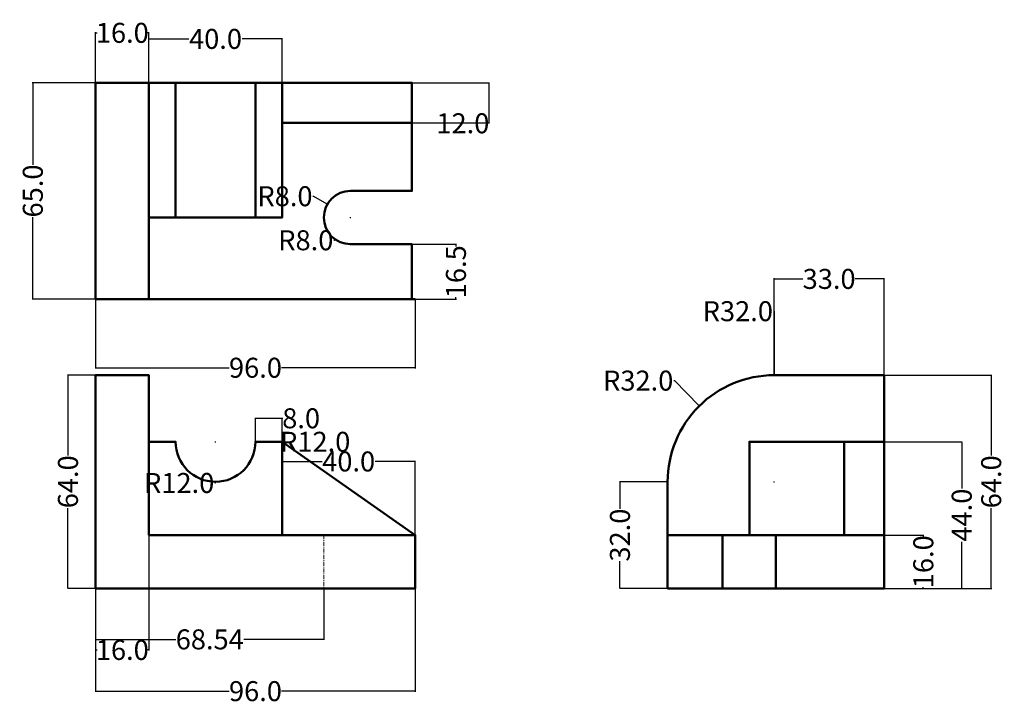
# Model space of a CAD drawing. Units: millimetres. Extents: x 2 to 298, y 17 to 222.
import ezdxf

# ---------------------------------------------------------------- set-up
doc = ezdxf.new("R2010")
doc.units = ezdxf.units.MM
doc.header["$MEASUREMENT"] = 0
doc.linetypes.add('CENTER', pattern=[2, 1.25, -0.25, 0.25, -0.25])
for name, color, linetype, lineweight in [('M-CNTR', 4, 'CENTER', 18), ('M-DIMS', 2, 'Continuous', 25), ('M-OUTL', 7, 'Continuous', 50)]:
    doc.layers.add(name, color=color, linetype=linetype, lineweight=lineweight)
doc.styles.get("Standard").update_dxf_attribs({"font": 'arial.ttf'})
doc.dimstyles.get("Standard").update_dxf_attribs({"dimtxt": 6, "dimasz": 0.18, "dimexe": 0.18, "dimexo": 0.0625, "dimgap": 0.09, "dimtad": 0, "dimtoh": 1, "dimdec": 1, "dimzin": 0, "dimdsep": 46, "dimtxsty": 'Standard', "dimcen": 0.09, "dimadec": 0, "dimazin": 0, "dimtfac": 1, "dimtdec": 1, "dimtofl": 0, "dimtmove": 0, "dimatfit": 3, "dimfxl": 1, "dimtolj": 1, "dimtzin": 0, "dimarcsym": 0})

# ---------------------------------------------------------------- blocks, each defined once
blk = doc.blocks.new('*D1')
at = {"layer": 'Defpoints', "color": 0, "transparency": 16777216}
for p in [(40.65, 218.17), (24.65, 203.2), (40.65, 203.2)]:
    blk.add_point(p, dxfattribs=at)
at = {"layer": 'M-DIMS', "color": 0, "lineweight": -2, "transparency": 16777216}
for p, q in [((24.65, 203.26), (24.65, 218.35)), ((24.83, 218.17), (25.06, 218.17)), ((40.47, 218.17), (40.24, 218.17)), ((40.65, 203.26), (40.65, 218.35))]:
    blk.add_line(p, q, dxfattribs=at)
at = {"layer": 'M-DIMS', "color": 0, "transparency": 16777216}
for points in [[(24.83, 218.2), (24.83, 218.14), (24.65, 218.17)], [(40.47, 218.2), (40.47, 218.14), (40.65, 218.17)]]:
    blk.add_solid(points, dxfattribs=at)
at = {"layer": 'M-DIMS', "color": 0, "transparency": 16777216, "insert": (32.65, 218.17), "char_height": 6, "attachment_point": 5}
blk.add_mtext('\\A1;16.0', dxfattribs=at)
blk = doc.blocks.new('*D2')
at = {"layer": 'Defpoints', "color": 0, "transparency": 16777216}
for p in [(80.65, 216.35), (40.65, 203.2), (80.65, 203.2)]:
    blk.add_point(p, dxfattribs=at)
at = {"layer": 'M-DIMS', "color": 0, "lineweight": -2, "transparency": 16777216}
for p, q in [((40.65, 203.26), (40.65, 216.53)), ((40.83, 216.35), (52.66, 216.35)), ((80.47, 216.35), (68.64, 216.35)), ((80.65, 203.26), (80.65, 216.53))]:
    blk.add_line(p, q, dxfattribs=at)
at = {"layer": 'M-DIMS', "color": 0, "transparency": 16777216}
for points in [[(40.83, 216.38), (40.83, 216.32), (40.65, 216.35)], [(80.47, 216.38), (80.47, 216.32), (80.65, 216.35)]]:
    blk.add_solid(points, dxfattribs=at)
at = {"layer": 'M-DIMS', "color": 0, "transparency": 16777216, "insert": (60.65, 216.35), "char_height": 6, "attachment_point": 5}
blk.add_mtext('\\A1;40.0', dxfattribs=at)
blk = doc.blocks.new('*D3')
at = {"layer": 'Defpoints', "color": 0, "transparency": 16777216}
for p in [(24.65, 203.2), (5.77, 138.2), (24.65, 138.2)]:
    blk.add_point(p, dxfattribs=at)
at = {"layer": 'M-DIMS', "color": 0, "lineweight": -2, "transparency": 16777216}
for p, q in [((24.59, 203.2), (5.59, 203.2)), ((5.77, 203.02), (5.77, 178.59)), ((5.77, 138.38), (5.77, 162.81)), ((24.59, 138.2), (5.59, 138.2))]:
    blk.add_line(p, q, dxfattribs=at)
at = {"layer": 'M-DIMS', "color": 0, "transparency": 16777216}
for points in [[(5.74, 203.02), (5.8, 203.02), (5.77, 203.2)], [(5.74, 138.38), (5.8, 138.38), (5.77, 138.2)]]:
    blk.add_solid(points, dxfattribs=at)
at = {"layer": 'M-DIMS', "color": 0, "transparency": 16777216, "insert": (5.77, 170.7), "char_height": 6, "attachment_point": 5, "rotation": 90}
blk.add_mtext('\\A1;65.0', dxfattribs=at)
blk = doc.blocks.new('*D4')
at = {"layer": 'Defpoints', "color": 0, "transparency": 16777216}
for p in [(24.65, 138.2), (120.65, 138.2), (120.65, 117.65)]:
    blk.add_point(p, dxfattribs=at)
at = {"layer": 'M-DIMS', "color": 0, "lineweight": -2, "transparency": 16777216}
for p, q in [((24.65, 138.14), (24.65, 117.47)), ((120.65, 138.14), (120.65, 117.47)), ((24.83, 117.65), (64.78, 117.65)), ((120.47, 117.65), (80.52, 117.65))]:
    blk.add_line(p, q, dxfattribs=at)
at = {"layer": 'M-DIMS', "color": 0, "transparency": 16777216}
for points in [[(24.83, 117.68), (24.83, 117.62), (24.65, 117.65)], [(120.47, 117.68), (120.47, 117.62), (120.65, 117.65)]]:
    blk.add_solid(points, dxfattribs=at)
at = {"layer": 'M-DIMS', "color": 0, "transparency": 16777216, "insert": (72.65, 117.65), "char_height": 6, "attachment_point": 5}
blk.add_mtext('\\A1;96.0', dxfattribs=at)
blk = doc.blocks.new('*D5')
at = {"layer": 'Defpoints', "color": 0, "transparency": 16777216}
for p in [(101.19, 162.73), (96.57, 156.2)]:
    blk.add_point(p, dxfattribs=at)
at = {"layer": 'M-DIMS', "color": 0, "lineweight": -2, "transparency": 16777216}
for p, q in [((101.1, 162.73), (101.28, 162.73)), ((101.19, 162.64), (101.19, 162.82)), ((96.18, 155.91), (96.36, 155.91)), ((96.36, 155.91), (96.47, 156.06))]:
    blk.add_line(p, q, dxfattribs=at)
at = {"layer": 'M-DIMS', "color": 0, "transparency": 16777216}
blk.add_solid([(96.44, 156.07), (96.49, 156.04), (96.57, 156.2)], dxfattribs=at)
at = {"layer": 'M-DIMS', "color": 0, "transparency": 16777216, "insert": (87.77, 155.91), "char_height": 6, "attachment_point": 5}
blk.add_mtext('\\A1;R8.0', dxfattribs=at)
blk = doc.blocks.new('*D6')
at = {"layer": 'Defpoints', "color": 0, "transparency": 16777216}
for p in [(119.65, 203.2), (119.65, 191.2), (142.72, 191.2)]:
    blk.add_point(p, dxfattribs=at)
at = {"layer": 'M-DIMS', "color": 0, "lineweight": -2, "transparency": 16777216}
for p, q in [((119.71, 203.2), (142.9, 203.2)), ((142.72, 203.02), (142.72, 191.38)), ((119.71, 191.2), (142.9, 191.2)), ((142.72, 191.02), (142.54, 191.02)), ((142.72, 191.2), (142.72, 191.02))]:
    blk.add_line(p, q, dxfattribs=at)
at = {"layer": 'M-DIMS', "color": 0, "transparency": 16777216}
for points in [[(142.69, 203.02), (142.75, 203.02), (142.72, 203.2)], [(142.69, 191.38), (142.75, 191.38), (142.72, 191.2)]]:
    blk.add_solid(points, dxfattribs=at)
at = {"layer": 'M-DIMS', "color": 0, "transparency": 16777216, "insert": (134.95, 191.02), "char_height": 6, "attachment_point": 5}
blk.add_mtext('\\A1;12.0', dxfattribs=at)
blk = doc.blocks.new('*D7')
at = {"layer": 'Defpoints', "color": 0, "transparency": 16777216}
for p in [(119.65, 154.73), (119.65, 138.2), (132.87, 138.2)]:
    blk.add_point(p, dxfattribs=at)
at = {"layer": 'M-DIMS', "color": 0, "lineweight": -2, "transparency": 16777216}
for p, q in [((119.71, 154.73), (133.05, 154.73)), ((132.87, 154.55), (132.87, 154.09)), ((119.71, 138.2), (133.05, 138.2)), ((132.87, 138.38), (132.87, 138.84))]:
    blk.add_line(p, q, dxfattribs=at)
at = {"layer": 'M-DIMS', "color": 0, "transparency": 16777216}
for points in [[(132.84, 154.55), (132.9, 154.55), (132.87, 154.73)], [(132.84, 138.38), (132.9, 138.38), (132.87, 138.2)]]:
    blk.add_solid(points, dxfattribs=at)
at = {"layer": 'M-DIMS', "color": 0, "transparency": 16777216, "insert": (132.87, 146.46), "char_height": 6, "attachment_point": 5, "rotation": 90}
blk.add_mtext('\\A1;16.5', dxfattribs=at)
blk = doc.blocks.new('*D8')
at = {"layer": 'Defpoints', "color": 0, "transparency": 16777216}
for p in [(24.65, 83.42), (40.65, 83.42), (40.65, 32.95)]:
    blk.add_point(p, dxfattribs=at)
at = {"layer": 'M-DIMS', "color": 0, "lineweight": -2, "transparency": 16777216}
for p, q in [((24.65, 83.35), (24.65, 32.77)), ((40.65, 83.35), (40.65, 32.77)), ((24.83, 32.95), (25.06, 32.95)), ((40.47, 32.95), (40.24, 32.95))]:
    blk.add_line(p, q, dxfattribs=at)
at = {"layer": 'M-DIMS', "color": 0, "transparency": 16777216}
for points in [[(24.83, 32.98), (24.83, 32.92), (24.65, 32.95)], [(40.47, 32.98), (40.47, 32.92), (40.65, 32.95)]]:
    blk.add_solid(points, dxfattribs=at)
at = {"layer": 'M-DIMS', "color": 0, "transparency": 16777216, "insert": (32.65, 32.95), "char_height": 6, "attachment_point": 5}
blk.add_mtext('\\A1;16.0', dxfattribs=at)
blk = doc.blocks.new('*D9')
at = {"layer": 'Defpoints', "color": 0, "transparency": 16777216}
for p in [(24.65, 115.42), (16.33, 51.42), (24.65, 51.42)]:
    blk.add_point(p, dxfattribs=at)
at = {"layer": 'M-DIMS', "color": 0, "lineweight": -2, "transparency": 16777216}
for p, q in [((24.59, 115.42), (16.15, 115.42)), ((16.33, 115.24), (16.33, 91.31)), ((16.33, 51.6), (16.33, 75.53)), ((24.59, 51.42), (16.15, 51.42))]:
    blk.add_line(p, q, dxfattribs=at)
at = {"layer": 'M-DIMS', "color": 0, "transparency": 16777216}
for points in [[(16.3, 115.24), (16.36, 115.24), (16.33, 115.42)], [(16.3, 51.6), (16.36, 51.6), (16.33, 51.42)]]:
    blk.add_solid(points, dxfattribs=at)
at = {"layer": 'M-DIMS', "color": 0, "transparency": 16777216, "insert": (16.33, 83.42), "char_height": 6, "attachment_point": 5, "rotation": 90}
blk.add_mtext('\\A1;64.0', dxfattribs=at)
blk = doc.blocks.new('*D10')
at = {"layer": 'Defpoints', "color": 0, "transparency": 16777216}
for p in [(60.65, 95.42), (60.65, 83.42)]:
    blk.add_point(p, dxfattribs=at)
at = {"layer": 'M-DIMS', "color": 0, "lineweight": -2, "transparency": 16777216}
for p, q in [((60.56, 95.42), (60.74, 95.42)), ((60.65, 95.33), (60.65, 95.51)), ((60.47, 83.06), (60.65, 83.06)), ((60.65, 83.06), (60.65, 83.24))]:
    blk.add_line(p, q, dxfattribs=at)
at = {"layer": 'M-DIMS', "color": 0, "transparency": 16777216}
blk.add_solid([(60.62, 83.24), (60.68, 83.24), (60.65, 83.42)], dxfattribs=at)
at = {"layer": 'M-DIMS', "color": 0, "transparency": 16777216, "insert": (49.73, 83.06), "char_height": 6, "attachment_point": 5}
blk.add_mtext('\\A1;R12.0', dxfattribs=at)
blk = doc.blocks.new('*D11')
at = {"layer": 'Defpoints', "color": 0, "transparency": 16777216}
for p in [(80.65, 102.48), (72.65, 95.42), (80.65, 95.42)]:
    blk.add_point(p, dxfattribs=at)
at = {"layer": 'M-DIMS', "color": 0, "lineweight": -2, "transparency": 16777216}
for p, q in [((72.65, 95.48), (72.65, 102.66)), ((72.83, 102.48), (80.47, 102.48)), ((80.65, 95.48), (80.65, 102.66)), ((80.65, 102.48), (80.83, 102.48))]:
    blk.add_line(p, q, dxfattribs=at)
at = {"layer": 'M-DIMS', "color": 0, "transparency": 16777216}
for points in [[(72.83, 102.51), (72.83, 102.45), (72.65, 102.48)], [(80.47, 102.51), (80.47, 102.45), (80.65, 102.48)]]:
    blk.add_solid(points, dxfattribs=at)
at = {"layer": 'M-DIMS', "color": 0, "transparency": 16777216, "insert": (86.37, 102.48), "char_height": 6, "attachment_point": 5}
blk.add_mtext('\\A1;8.0', dxfattribs=at)
blk = doc.blocks.new('*D12')
at = {"layer": 'Defpoints', "color": 0, "transparency": 16777216}
for p in [(120.65, 89.52), (80.65, 67.42), (120.65, 67.42)]:
    blk.add_point(p, dxfattribs=at)
at = {"layer": 'M-DIMS', "color": 0, "lineweight": -2, "transparency": 16777216}
for p, q in [((80.65, 67.48), (80.65, 89.7)), ((80.83, 89.52), (92.66, 89.52)), ((120.47, 89.52), (108.64, 89.52)), ((120.65, 67.48), (120.65, 89.7))]:
    blk.add_line(p, q, dxfattribs=at)
at = {"layer": 'M-DIMS', "color": 0, "transparency": 16777216}
for points in [[(80.83, 89.55), (80.83, 89.49), (80.65, 89.52)], [(120.47, 89.55), (120.47, 89.49), (120.65, 89.52)]]:
    blk.add_solid(points, dxfattribs=at)
at = {"layer": 'M-DIMS', "color": 0, "transparency": 16777216, "insert": (100.65, 89.52), "char_height": 6, "attachment_point": 5}
blk.add_mtext('\\A1;40.0', dxfattribs=at)
blk = doc.blocks.new('*D13')
at = {"layer": 'Defpoints', "color": 0, "transparency": 16777216}
for p in [(24.65, 51.42), (120.65, 51.42), (120.65, 20.58)]:
    blk.add_point(p, dxfattribs=at)
at = {"layer": 'M-DIMS', "color": 0, "lineweight": -2, "transparency": 16777216}
for p, q in [((24.65, 51.35), (24.65, 20.4)), ((120.65, 51.35), (120.65, 20.4)), ((24.83, 20.58), (64.78, 20.58)), ((120.47, 20.58), (80.52, 20.58))]:
    blk.add_line(p, q, dxfattribs=at)
at = {"layer": 'M-DIMS', "color": 0, "transparency": 16777216}
for points in [[(24.83, 20.61), (24.83, 20.55), (24.65, 20.58)], [(120.47, 20.61), (120.47, 20.55), (120.65, 20.58)]]:
    blk.add_solid(points, dxfattribs=at)
at = {"layer": 'M-DIMS', "color": 0, "transparency": 16777216, "insert": (72.65, 20.58), "char_height": 6, "attachment_point": 5}
blk.add_mtext('\\A1;96.0', dxfattribs=at)
blk = doc.blocks.new('*D14')
at = {"layer": 'Defpoints', "color": 0, "transparency": 16777216}
for p in [(261.46, 144.31), (228.46, 115.42), (261.46, 115.42)]:
    blk.add_point(p, dxfattribs=at)
at = {"layer": 'M-DIMS', "color": 0, "lineweight": -2, "transparency": 16777216}
for p, q in [((228.46, 115.48), (228.46, 144.49)), ((228.64, 144.31), (237.09, 144.31)), ((261.28, 144.31), (252.83, 144.31)), ((261.46, 115.48), (261.46, 144.49))]:
    blk.add_line(p, q, dxfattribs=at)
at = {"layer": 'M-DIMS', "color": 0, "transparency": 16777216}
for points in [[(228.64, 144.34), (228.64, 144.28), (228.46, 144.31)], [(261.28, 144.34), (261.28, 144.28), (261.46, 144.31)]]:
    blk.add_solid(points, dxfattribs=at)
at = {"layer": 'M-DIMS', "color": 0, "transparency": 16777216, "insert": (244.96, 144.31), "char_height": 6, "attachment_point": 5}
blk.add_mtext('\\A1;33.0', dxfattribs=at)
blk = doc.blocks.new('*D15')
at = {"layer": 'Defpoints', "color": 0, "transparency": 16777216}
for p in [(196.46, 83.42), (182.13, 51.42), (196.46, 51.42)]:
    blk.add_point(p, dxfattribs=at)
at = {"layer": 'M-DIMS', "color": 0, "lineweight": -2, "transparency": 16777216}
for p, q in [((196.39, 83.42), (181.95, 83.42)), ((182.13, 83.24), (182.13, 75.29)), ((182.13, 51.6), (182.13, 59.55)), ((196.39, 51.42), (181.95, 51.42))]:
    blk.add_line(p, q, dxfattribs=at)
at = {"layer": 'M-DIMS', "color": 0, "transparency": 16777216}
for points in [[(182.1, 83.24), (182.16, 83.24), (182.13, 83.42)], [(182.1, 51.6), (182.16, 51.6), (182.13, 51.42)]]:
    blk.add_solid(points, dxfattribs=at)
at = {"layer": 'M-DIMS', "color": 0, "transparency": 16777216, "insert": (182.13, 67.42), "char_height": 6, "attachment_point": 5, "rotation": 90}
blk.add_mtext('\\A1;32.0', dxfattribs=at)
blk = doc.blocks.new('*D16')
at = {"layer": 'Defpoints', "color": 0, "transparency": 16777216}
for p in [(261.46, 115.42), (261.46, 51.42), (293.64, 51.42)]:
    blk.add_point(p, dxfattribs=at)
at = {"layer": 'M-DIMS', "color": 0, "lineweight": -2, "transparency": 16777216}
for p, q in [((261.52, 115.42), (293.82, 115.42)), ((293.64, 115.24), (293.64, 91.31)), ((293.64, 51.6), (293.64, 75.53)), ((261.52, 51.42), (293.82, 51.42))]:
    blk.add_line(p, q, dxfattribs=at)
at = {"layer": 'M-DIMS', "color": 0, "transparency": 16777216}
for points in [[(293.61, 115.24), (293.67, 115.24), (293.64, 115.42)], [(293.61, 51.6), (293.67, 51.6), (293.64, 51.42)]]:
    blk.add_solid(points, dxfattribs=at)
at = {"layer": 'M-DIMS', "color": 0, "transparency": 16777216, "insert": (293.64, 83.42), "char_height": 6, "attachment_point": 5, "rotation": 90}
blk.add_mtext('\\A1;64.0', dxfattribs=at)
blk = doc.blocks.new('*D17')
at = {"layer": 'Defpoints', "color": 0, "transparency": 16777216}
for p in [(261.46, 95.42), (261.46, 51.42), (284.79, 51.42)]:
    blk.add_point(p, dxfattribs=at)
at = {"layer": 'M-DIMS', "color": 0, "lineweight": -2, "transparency": 16777216}
for p, q in [((261.52, 95.42), (284.97, 95.42)), ((284.79, 95.24), (284.79, 81.41)), ((284.79, 51.6), (284.79, 65.42)), ((261.52, 51.42), (284.97, 51.42))]:
    blk.add_line(p, q, dxfattribs=at)
at = {"layer": 'M-DIMS', "color": 0, "transparency": 16777216}
for points in [[(284.76, 95.24), (284.82, 95.24), (284.79, 95.42)], [(284.76, 51.6), (284.82, 51.6), (284.79, 51.42)]]:
    blk.add_solid(points, dxfattribs=at)
at = {"layer": 'M-DIMS', "color": 0, "transparency": 16777216, "insert": (284.79, 73.42), "char_height": 6, "attachment_point": 5, "rotation": 90}
blk.add_mtext('\\A1;44.0', dxfattribs=at)
blk = doc.blocks.new('*D18')
at = {"layer": 'Defpoints', "color": 0, "transparency": 16777216}
for p in [(261.46, 67.42), (261.46, 51.42), (273.25, 51.42)]:
    blk.add_point(p, dxfattribs=at)
at = {"layer": 'M-DIMS', "color": 0, "lineweight": -2, "transparency": 16777216}
for p, q in [((261.52, 67.42), (273.43, 67.42)), ((273.25, 67.24), (273.25, 67.01)), ((261.52, 51.42), (273.43, 51.42)), ((273.25, 51.6), (273.25, 51.83))]:
    blk.add_line(p, q, dxfattribs=at)
at = {"layer": 'M-DIMS', "color": 0, "transparency": 16777216}
for points in [[(273.22, 67.24), (273.28, 67.24), (273.25, 67.42)], [(273.22, 51.6), (273.28, 51.6), (273.25, 51.42)]]:
    blk.add_solid(points, dxfattribs=at)
at = {"layer": 'M-DIMS', "color": 0, "transparency": 16777216, "insert": (273.25, 59.42), "char_height": 6, "attachment_point": 5, "rotation": 90}
blk.add_mtext('\\A1;16.0', dxfattribs=at)
blk = doc.blocks.new('*D19')
at = {"layer": 'Defpoints', "color": 0, "transparency": 16777216}
for p in [(206, 106.21), (228.46, 83.42)]:
    blk.add_point(p, dxfattribs=at)
at = {"layer": 'M-DIMS', "color": 0, "lineweight": -2, "transparency": 16777216}
for p, q in [((198.36, 113.79), (198.54, 113.79)), ((198.54, 113.79), (205.87, 106.34)), ((228.37, 83.42), (228.55, 83.42)), ((228.46, 83.33), (228.46, 83.51))]:
    blk.add_line(p, q, dxfattribs=at)
at = {"layer": 'M-DIMS', "color": 0, "transparency": 16777216}
blk.add_solid([(205.89, 106.36), (205.85, 106.32), (206, 106.21)], dxfattribs=at)
at = {"layer": 'M-DIMS', "color": 0, "transparency": 16777216, "insert": (187.61, 113.79), "char_height": 6, "attachment_point": 5}
blk.add_mtext('\\A1;R32.0', dxfattribs=at)
blk = doc.blocks.new('*D20')
at = {"layer": 'Defpoints', "color": 0, "transparency": 16777216}
for p in [(24.65, 51.42), (93.19, 51.42), (93.19, 36.12)]:
    blk.add_point(p, dxfattribs=at)
at = {"layer": 'M-DIMS', "color": 0, "lineweight": -2, "transparency": 16777216}
for p, q in [((24.65, 51.35), (24.65, 35.94)), ((93.19, 51.35), (93.19, 35.94)), ((24.83, 36.12), (48.7, 36.12)), ((93.01, 36.12), (69.14, 36.12))]:
    blk.add_line(p, q, dxfattribs=at)
at = {"layer": 'M-DIMS', "color": 0, "transparency": 16777216}
for points in [[(24.83, 36.15), (24.83, 36.09), (24.65, 36.12)], [(93.01, 36.15), (93.01, 36.09), (93.19, 36.12)]]:
    blk.add_solid(points, dxfattribs=at)
at = {"layer": 'M-DIMS', "color": 0, "transparency": 16777216, "insert": (58.92, 36.12), "char_height": 6, "attachment_point": 5}
blk.add_mtext('\\A1;68.54', dxfattribs=at)
blk = doc.blocks.new('*D21')
at = {"layer": 'Defpoints', "color": 0, "transparency": 16777216}
for p in [(228.46, 115.42), (228.46, 83.42)]:
    blk.add_point(p, dxfattribs=at)
at = {"layer": 'M-DIMS', "color": 0, "lineweight": -2, "transparency": 16777216}
for p, q in [((228.28, 134.62), (228.46, 134.62)), ((228.46, 134.62), (228.46, 115.6)), ((228.37, 83.42), (228.55, 83.42)), ((228.46, 83.33), (228.46, 83.51))]:
    blk.add_line(p, q, dxfattribs=at)
at = {"layer": 'M-DIMS', "color": 0, "transparency": 16777216}
blk.add_solid([(228.49, 115.6), (228.43, 115.6), (228.46, 115.42)], dxfattribs=at)
at = {"layer": 'M-DIMS', "color": 0, "transparency": 16777216, "insert": (217.53, 134.62), "char_height": 6, "attachment_point": 5}
blk.add_mtext('\\A1;R32.0', dxfattribs=at)
blk = doc.blocks.new('*D22')
at = {"layer": 'Defpoints', "color": 0, "transparency": 16777216}
for p in [(60.65, 95.42), (72.65, 95.42)]:
    blk.add_point(p, dxfattribs=at)
at = {"layer": 'M-DIMS', "color": 0, "lineweight": -2, "transparency": 16777216}
for p, q in [((60.56, 95.42), (60.74, 95.42)), ((60.65, 95.33), (60.65, 95.51)), ((79.85, 95.42), (72.83, 95.42))]:
    blk.add_line(p, q, dxfattribs=at)
at = {"layer": 'M-DIMS', "color": 0, "transparency": 16777216}
blk.add_solid([(72.83, 95.45), (72.83, 95.39), (72.65, 95.42)], dxfattribs=at)
at = {"layer": 'M-DIMS', "color": 0, "transparency": 16777216, "insert": (90.59, 95.42), "char_height": 6, "attachment_point": 5}
blk.add_mtext('\\A1;R12.0', dxfattribs=at)
blk = doc.blocks.new('*D23')
at = {"layer": 'Defpoints', "color": 0, "transparency": 16777216}
for p in [(94.26, 166.73), (101.19, 162.73)]:
    blk.add_point(p, dxfattribs=at)
at = {"layer": 'M-DIMS', "color": 0, "lineweight": -2, "transparency": 16777216}
for p, q in [((89.92, 169.13), (90.1, 169.13)), ((90.1, 169.13), (94.11, 166.82)), ((101.1, 162.73), (101.28, 162.73)), ((101.19, 162.64), (101.19, 162.82))]:
    blk.add_line(p, q, dxfattribs=at)
at = {"layer": 'M-DIMS', "color": 0, "transparency": 16777216}
blk.add_solid([(94.12, 166.84), (94.09, 166.79), (94.26, 166.73)], dxfattribs=at)
at = {"layer": 'M-DIMS', "color": 0, "transparency": 16777216, "insert": (81.51, 169.13), "char_height": 6, "attachment_point": 5}
blk.add_mtext('\\A1;R8.0', dxfattribs=at)

msp = doc.modelspace()

# ---------------------------------------------------------------- linework, layer by layer
at = {"layer": 'M-CNTR'}
msp.add_line((93.192, 67.417), (93.192, 51.417), dxfattribs=at)
at = {"layer": 'M-OUTL'}
for p, q in [((40.649, 203.198), (40.649, 138.198)), ((72.649, 203.198), (72.649, 162.732)), ((119.649, 191.198), (80.649, 191.198)), ((249.456, 95.417), (249.456, 67.417)), ((196.456, 67.417), (261.456, 67.417)), ((212.956, 51.417), (212.956, 67.417)), ((228.956, 51.417), (228.956, 67.417))]:
    msp.add_line(p, q, dxfattribs=at)
for points in [[(120.649, 138.198), (24.649, 138.198), (24.649, 203.198), (119.649, 203.198), (119.649, 170.732), (101.192, 170.732, 1), (101.192, 154.732), (119.649, 154.732), (119.649, 138.198)], [(40.649, 95.417), (48.649, 95.417, 1), (72.649, 95.417), (80.649, 95.417)]]:
    msp.add_lwpolyline(points, format="xyb", dxfattribs=at)
for points in [[(40.649, 162.732), (48.649, 162.732), (80.649, 162.732), (80.649, 203.198)], [(48.649, 203.198), (48.649, 185.432), (48.649, 170.732), (48.649, 162.732)], [(80.649, 67.417), (80.649, 95.417), (120.649, 67.417), (120.649, 51.417), (24.649, 51.417), (24.649, 115.417), (40.649, 115.417), (40.649, 67.417), (120.649, 67.417)], [(261.456, 95.417), (236.497, 95.417), (220.997, 95.417), (220.997, 67.417)]]:
    msp.add_lwpolyline(points, dxfattribs=at)
msp.add_lwpolyline([(196.456, 51.417), (196.456, 83.417, -0.4142136), (228.456, 115.417), (261.456, 115.417), (261.456, 51.417)], format="xyb", close=True, dxfattribs=at)

# ---------------------------------------------------------------- dimensions: what is measured, and where the dimension line sits
at = {"layer": 'M-DIMS'}
for base, p1, p2, override, picture, middle in [((40.649, 218.173), (24.649, 203.198), (40.649, 203.198), {"dimclrd": 0, "dimclre": 0, "dimclrt": 0}, '*D1', (32.649, 218.173)), ((80.649, 216.351), (40.649, 203.198), (80.649, 203.198), {"dimclrd": 0, "dimclre": 0, "dimclrt": 0}, '*D2', (60.649, 216.351)), ((261.456, 144.313), (228.456, 115.417), (261.456, 115.417), {"dimclrd": 0, "dimclre": 0, "dimclrt": 0}, '*D14', (244.956, 144.313)), ((120.649, 117.651), (24.649, 138.198), (120.649, 138.198), {"dimclrd": 0, "dimclre": 0, "dimclrt": 0}, '*D4', (72.649, 117.651)), ((80.649, 102.478), (72.649, 95.417), (80.649, 95.417), {"dimclrd": 0, "dimclre": 0, "dimclrt": 0}, '*D11', (86.374, 102.478)), ((120.649, 89.515), (80.649, 67.417), (120.649, 67.417), {"dimclrd": 0, "dimclre": 0, "dimclrt": 0}, '*D12', (100.649, 89.515)), ((40.649, 32.95), (24.649, 83.417), (40.649, 83.417), {"dimclrd": 0, "dimclre": 0, "dimclrt": 0}, '*D8', (32.649, 32.95)), ((120.649, 20.576), (24.649, 51.417), (120.649, 51.417), {"dimclrd": 0, "dimclre": 0, "dimclrt": 0}, '*D13', (72.649, 20.576)), ((93.192, 36.117), (24.649, 51.417), (93.192, 51.417), {"dimdec": 2, "dimlfac": 1, "dimrnd": 0, "dimzin": 0, "dimdsep": 46, "dimlunit": 2}, '*D20', (58.921, 36.117))]:
    dim = msp.add_linear_dim(base=base, p1=p1, p2=p2, dimstyle='Standard', override=override, dxfattribs=at)
    dim.commit()
    dim.dimension.update_dxf_attribs({"geometry": picture, "text_midpoint": middle})
for base, p1, p2, picture, middle in [((5.768, 138.198), (24.649, 203.198), (24.649, 138.198), '*D3', (5.768, 170.698)), ((142.724, 191.198), (119.649, 203.198), (119.649, 191.198), '*D6', (134.954, 191.018)), ((132.869, 138.198), (119.649, 154.732), (119.649, 138.198), '*D7', (132.869, 146.465)), ((16.327, 51.417), (24.649, 115.417), (24.649, 51.417), '*D9', (16.327, 83.417)), ((293.644, 51.417), (261.456, 115.417), (261.456, 51.417), '*D16', (293.644, 83.417)), ((284.794, 51.417), (261.456, 95.417), (261.456, 51.417), '*D17', (284.794, 73.417)), ((182.127, 51.417), (196.456, 83.417), (196.456, 51.417), '*D15', (182.127, 67.417)), ((273.246, 51.417), (261.456, 67.417), (261.456, 51.417), '*D18', (273.246, 59.417))]:
    dim = msp.add_linear_dim(base=base, p1=p1, p2=p2, angle=90, dimstyle='Standard', override={"dimclrd": 0, "dimclre": 0, "dimclrt": 0}, dxfattribs=at)
    dim.commit()
    dim.dimension.update_dxf_attribs({"geometry": picture, "text_midpoint": middle})
for center, mpoint, override, picture, middle in [((101.192, 162.732), (94.262, 166.729), {"dimdec": 1, "dimlfac": 1, "dimrnd": 0, "dimzin": 0, "dimdsep": 46, "dimlunit": 2}, '*D23', (81.512, 169.127)), ((228.456, 83.417), (228.456, 115.417), {"dimdec": 1, "dimlfac": 1, "dimrnd": 0, "dimzin": 0, "dimdsep": 46, "dimlunit": 2}, '*D21', (217.532, 134.617)), ((228.456, 83.417), (205.997, 106.212), {"dimclrd": 0, "dimclre": 0, "dimclrt": 0}, '*D19', (187.612, 113.785)), ((60.649, 95.417), (72.649, 95.417), {"dimdec": 1, "dimlfac": 1, "dimrnd": 0, "dimzin": 0, "dimdsep": 46, "dimlunit": 2}, '*D22', (79.849, 95.417))]:
    dim = msp.add_radius_dim(center=center, mpoint=mpoint, dimstyle='Standard', override=override, dxfattribs=at)
    dim.commit()
    dim.dimension.update_dxf_attribs({"geometry": picture, "text_midpoint": middle, "dimtype": 164})
for center, mpoint, picture, middle in [((101.192, 162.732), (96.57, 156.203), '*D5', (87.769, 155.909)), ((60.649, 95.417), (60.649, 83.417), '*D10', (49.725, 83.057))]:
    dim = msp.add_radius_dim(center=center, mpoint=mpoint, dimstyle='Standard', override={"dimclrd": 0, "dimclre": 0, "dimclrt": 0}, dxfattribs=at)
    dim.commit()
    dim.dimension.update_dxf_attribs({"geometry": picture, "text_midpoint": middle})

doc.saveas('drawing.dxf')
